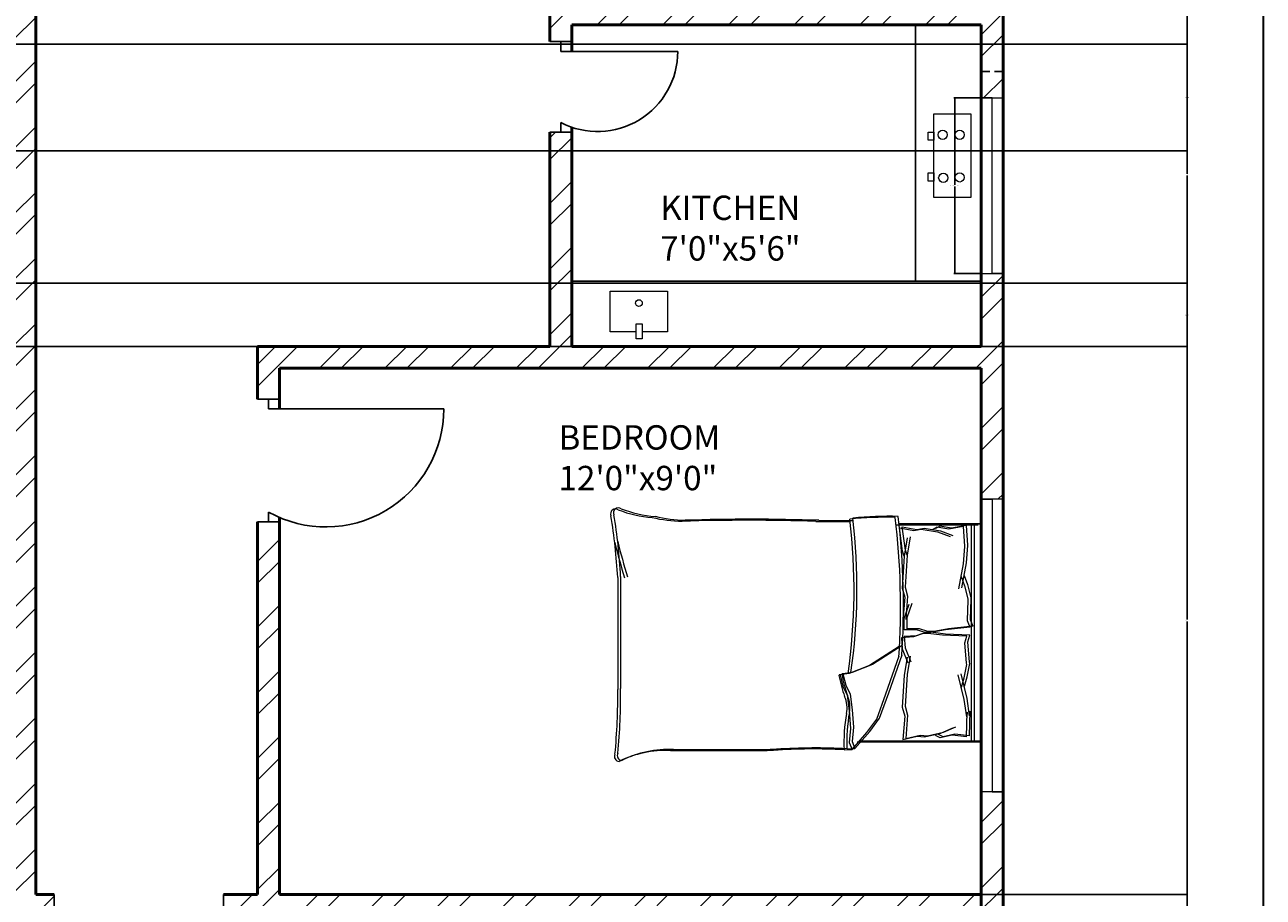
# Model space of a CAD drawing. Units: inches. Extents: x 2129 to 2642, y 1542 to 2414.
# Tile 4 of 9: x 2388 to 2642, y 1828 to 2007. Entities that reach past the tile are written whole.
import ezdxf

# ---------------------------------------------------------------- set-up
doc = ezdxf.new("R2010")
doc.units = ezdxf.units.IN
for name, color, linetype, lineweight in [('A-ANNO-DIMS', 2, 'Continuous', 18), ('A-ANNO-TTLB', 7, 'Continuous', 35), ('A-AREA-IDEN', 7, 'Continuous', 18), ('A-DOOR', 3, 'Continuous', 25), ('A-EQPM', 8, 'Continuous', 18), ('A-FLOR-CASE', 8, 'Continuous', 25), ('A-FLOR-FIXT', 9, 'Continuous', 18), ('A-FURN', 8, 'Continuous', 18), ('A-GLAZ', 4, 'Continuous', 18), ('A-WALL', 7, 'Continuous', 50), ('A-WALL-PATT', 252, 'Continuous', 13)]:
    doc.layers.add(name, color=color, linetype=linetype, lineweight=lineweight)
doc.styles.get("Standard").update_dxf_attribs({"font": 'arial.ttf'})
doc.dimstyles.get("Standard").update_dxf_attribs({"dimtxt": 0.18, "dimasz": 0.18, "dimexe": 0.18, "dimexo": 0.0625, "dimgap": 0.09, "dimtad": 0, "dimtih": 1, "dimtoh": 1, "dimdec": 4, "dimzin": 0, "dimdsep": 46, "dimtxsty": 'Standard', "dimcen": 0.09, "dimadec": 0, "dimazin": 0, "dimtfac": 1, "dimtdec": 4, "dimtofl": 0, "dimtmove": 0, "dimatfit": 3, "dimfxl": 1, "dimtolj": 1, "dimtzin": 0, "dimarcsym": 0})

# ---------------------------------------------------------------- blocks, each defined once
blk = doc.blocks.new('BED-DOUBLE')
for p, q in [((3.24, 59.14), (3.24, 76.05)), ((3.24, 74.61), (47.87, 74.61)), ((3.25, 59.14), (3.25, 76.05)), ((3.25, 74.61), (47.87, 74.61)), ((48.08, 76.05), (3.46, 76.05)), ((3.46, 58.54), (3.46, 75.45)), ((3.46, 58.54), (3.46, 75.45)), ((3.46, 74.02), (48.08, 74.02)), ((3.46, 74.02), (48.08, 74.02)), ((15.76, 73.22), (18.46, 73.9)), ((15.76, 73.22), (18.46, 73.9)), ((18.46, 73.9), (18.76, 73.9)), ((18.46, 73.9), (18.76, 73.9)), ((18.76, 73.9), (22.91, 73.76)), ((18.76, 73.9), (22.91, 73.76)), ((22.91, 73.76), (24.26, 74.3)), ((22.91, 73.76), (24.26, 74.3)), ((23.12, 73.16), (24.47, 73.7)), ((23.12, 73.16), (24.47, 73.7)), ((24.26, 74.3), (24.8, 69.31)), ((24.26, 74.3), (24.8, 69.31)), ((24.47, 73.7), (25.01, 68.71)), ((24.47, 73.7), (25.01, 68.71)), ((26.12, 73.72), (25.9, 68.7)), ((26.12, 73.72), (25.9, 68.7)), ((27.5, 73.27), (26.12, 73.72)), ((27.5, 73.27), (26.12, 73.72)), ((46.79, 73.66), (41.75, 73.75)), ((41.75, 73.75), (42.68, 73.67)), ((46.79, 73.66), (41.75, 73.75)), ((41.75, 73.75), (42.68, 73.67)), ((47.87, 76.05), (47.87, 51.2)), ((47.87, 76.05), (47.87, 51.2)), ((48.08, 76.05), (48.08, 75.45)), ((48.08, 75.45), (48.08, 50.6)), ((48.08, 75.45), (48.08, 50.6)), ((3.64, 72.93), (7.64, 73.24)), ((3.64, 72.93), (7.64, 73.24)), ((3.64, 72.95), (4.18, 69.98)), ((3.64, 72.95), (4.18, 69.98)), ((3.85, 72.33), (7.85, 72.64)), ((3.85, 72.33), (7.85, 72.64)), ((3.85, 72.35), (4.39, 69.38)), ((3.85, 72.35), (4.39, 69.38)), ((7.64, 73.24), (7.74, 73.22)), ((7.64, 73.24), (7.74, 73.22)), ((7.74, 73.22), (11.31, 72.95)), ((7.74, 73.22), (11.31, 72.95)), ((7.85, 72.64), (7.95, 72.62)), ((7.85, 72.64), (7.95, 72.62)), ((7.95, 72.62), (11.52, 72.35)), ((7.95, 72.62), (11.52, 72.35)), ((11.31, 72.95), (16.44, 72.01)), ((11.31, 72.95), (16.44, 72.01)), ((11.52, 72.35), (16.65, 71.41)), ((11.52, 72.35), (16.65, 71.41)), ((13.87, 72.55), (15.76, 73.22)), ((13.87, 72.55), (15.76, 73.22)), ((14.08, 71.95), (15.97, 72.62)), ((14.08, 71.95), (15.97, 72.62)), ((15.97, 72.62), (18.67, 73.3)), ((15.97, 72.62), (18.67, 73.3)), ((18.67, 73.3), (18.97, 73.3)), ((18.67, 73.3), (18.97, 73.3)), ((18.97, 73.3), (23.12, 73.16)), ((18.97, 73.3), (23.12, 73.16)), ((26.34, 73.12), (26.11, 68.1)), ((26.34, 73.12), (26.11, 68.1)), ((27.72, 72.67), (26.34, 73.12)), ((27.72, 72.67), (26.34, 73.12)), ((31.64, 73.66), (27.5, 73.27)), ((31.64, 73.66), (27.5, 73.27)), ((31.85, 73.06), (27.72, 72.67)), ((31.85, 73.06), (27.72, 72.67)), ((31.94, 73.68), (31.64, 73.66)), ((31.94, 73.68), (31.64, 73.66)), ((32.15, 73.08), (31.85, 73.06)), ((32.15, 73.08), (31.85, 73.06)), ((34.68, 73.17), (31.94, 73.68)), ((34.67, 73.17), (31.94, 73.68)), ((34.89, 72.58), (32.15, 73.08)), ((34.89, 72.58), (32.15, 73.08)), ((39.14, 73.18), (34.08, 71.92)), ((39.14, 73.18), (34.08, 71.92)), ((39.35, 72.58), (34.29, 71.32)), ((39.35, 72.58), (34.29, 71.32)), ((36.6, 72.62), (34.67, 73.17)), ((36.6, 72.62), (34.68, 73.17)), ((36.82, 72.02), (34.89, 72.58)), ((36.82, 72.02), (34.89, 72.58)), ((42.68, 73.67), (39.14, 73.18)), ((42.68, 73.67), (39.14, 73.18)), ((42.9, 73.08), (39.35, 72.58)), ((42.9, 73.08), (39.35, 72.58)), ((47.01, 73.06), (41.96, 73.15)), ((41.96, 73.15), (42.9, 73.08)), ((47.01, 73.06), (41.96, 73.15)), ((41.96, 73.15), (42.9, 73.08)), ((46.79, 73.66), (46.44, 70.66)), ((46.79, 73.66), (46.44, 70.66)), ((47.01, 73.06), (46.65, 70.06)), ((47.01, 73.06), (46.65, 70.06)), ((4.18, 69.98), (3.77, 67.55)), ((4.18, 69.98), (3.77, 67.55)), ((4.39, 69.38), (3.98, 66.95)), ((4.39, 69.38), (3.99, 66.95)), ((4.72, 67.69), (5.66, 70.25)), ((4.72, 67.69), (5.66, 70.25)), ((4.93, 67.09), (5.87, 69.65)), ((4.93, 67.09), (5.87, 69.65)), ((24.8, 69.31), (25.34, 66.34)), ((24.8, 69.31), (25.34, 66.34)), ((25.01, 68.71), (25.55, 65.74)), ((25.01, 68.71), (25.55, 65.74)), ((25.9, 68.7), (25.54, 65.7)), ((25.9, 68.7), (25.54, 65.7)), ((46.04, 68.34), (44.94, 70.84)), ((46.04, 68.34), (44.94, 70.84)), ((46.26, 67.74), (45.15, 70.24)), ((46.26, 67.74), (45.15, 70.24)), ((46.44, 70.66), (46.99, 68.26)), ((46.44, 70.66), (46.99, 68.26)), ((46.65, 70.06), (47.21, 67.66)), ((46.65, 70.06), (47.21, 67.66)), ((3.77, 67.55), (4.31, 66.61)), ((3.77, 67.55), (4.31, 66.61)), ((3.98, 66.95), (4.52, 66.01)), ((3.99, 66.95), (4.53, 66.01)), ((4.18, 64.31), (4.72, 67.69)), ((4.18, 64.31), (4.72, 67.69)), ((4.39, 63.71), (4.93, 67.09)), ((4.39, 63.71), (4.93, 67.09)), ((25.34, 66.34), (25.34, 65.12)), ((25.34, 66.34), (25.34, 65.12)), ((26.11, 68.1), (25.76, 65.11)), ((26.11, 68.1), (25.76, 65.11)), ((46.79, 65), (46.04, 68.34)), ((46.79, 65), (46.04, 68.34)), ((47.01, 64.41), (46.26, 67.74)), ((47.01, 64.41), (46.26, 67.74)), ((46.99, 68.26), (46.51, 67.28)), ((46.99, 68.26), (46.51, 67.28)), ((47.21, 67.66), (46.73, 66.69)), ((47.21, 67.66), (46.73, 66.69)), ((4.45, 62.82), (4.18, 64.31)), ((4.45, 62.82), (4.18, 64.31)), ((4.66, 62.23), (4.39, 63.71)), ((4.66, 62.23), (4.39, 63.71)), ((25.34, 65.12), (24.8, 63.36)), ((25.34, 65.12), (24.8, 63.36)), ((25.55, 64.52), (25.01, 62.77)), ((25.55, 64.52), (25.01, 62.77)), ((25.54, 65.7), (25.62, 64.49)), ((25.54, 65.7), (25.62, 64.49)), ((25.55, 65.74), (25.55, 64.52)), ((25.55, 65.74), (25.55, 64.52)), ((25.62, 64.49), (26.27, 62.77)), ((25.62, 64.49), (26.27, 62.77)), ((25.76, 65.11), (25.83, 63.89)), ((25.76, 65.11), (25.83, 63.89)), ((25.83, 63.89), (26.48, 62.18)), ((25.83, 63.89), (26.48, 62.18)), ((46.62, 63.5), (46.79, 65)), ((46.62, 63.5), (46.79, 65)), ((46.83, 62.91), (47.01, 64.41)), ((46.83, 62.91), (47.01, 64.41)), ((3.91, 59.85), (4.45, 62.82)), ((3.91, 59.85), (4.45, 62.82)), ((4.12, 59.26), (4.66, 62.23)), ((4.12, 59.26), (4.66, 62.23)), ((5.96, 61.45), (9.72, 60.83)), ((5.96, 61.45), (9.72, 60.83)), ((22.51, 60.86), (19.57, 61.88)), ((22.51, 60.86), (19.57, 61.88)), ((22.72, 60.26), (19.78, 61.28)), ((22.72, 60.26), (19.78, 61.28)), ((24.8, 63.36), (24.8, 60.86)), ((24.8, 63.36), (24.8, 60.86)), ((25.01, 62.77), (25.01, 60.26)), ((25.01, 62.77), (25.01, 60.26)), ((26.27, 62.77), (26.42, 60.27)), ((26.27, 62.77), (26.42, 60.27)), ((26.48, 62.18), (26.64, 59.68)), ((26.48, 62.18), (26.64, 59.68)), ((28.71, 60.42), (31.58, 61.62)), ((28.71, 60.42), (31.58, 61.62)), ((28.93, 59.82), (31.79, 61.02)), ((28.93, 59.82), (31.79, 61.02)), ((30.41, 61.45), (34.17, 60.83)), ((30.41, 61.45), (34.17, 60.83)), ((47.34, 60.57), (46.62, 63.5)), ((47.34, 60.57), (46.62, 63.5)), ((47.55, 59.98), (46.83, 62.91)), ((47.55, 59.98), (46.83, 62.91)), ((8.67, 60.53), (3.91, 59.85)), ((8.67, 60.53), (3.91, 59.85)), ((8.88, 59.93), (4.12, 59.26)), ((8.88, 59.93), (4.12, 59.26)), ((6.17, 60.86), (9.94, 60.23)), ((6.17, 60.86), (9.94, 60.23)), ((9.72, 60.83), (8.67, 60.53)), ((9.72, 60.83), (8.67, 60.53)), ((9.94, 60.23), (8.88, 59.93)), ((9.94, 60.23), (8.88, 59.93)), ((9.72, 60.83), (16.27, 60.43)), ((9.72, 60.83), (16.27, 60.43)), ((9.94, 60.23), (16.48, 59.83)), ((9.94, 60.23), (16.48, 59.83)), ((16.27, 60.43), (18.1, 60.95)), ((16.27, 60.43), (18.1, 60.95)), ((16.48, 59.83), (18.31, 60.35)), ((16.48, 59.83), (18.31, 60.35)), ((18.1, 60.95), (22.89, 60.57)), ((18.1, 60.95), (22.89, 60.57)), ((18.31, 60.35), (23.11, 59.98)), ((18.31, 60.35), (23.1, 59.98)), ((24.8, 60.86), (22.51, 60.86)), ((24.8, 60.86), (22.51, 60.86)), ((25.01, 60.26), (22.72, 60.26)), ((25.01, 60.26), (22.72, 60.26)), ((26.42, 60.27), (28.71, 60.42)), ((26.42, 60.27), (28.71, 60.42)), ((26.64, 59.68), (28.93, 59.82)), ((26.64, 59.68), (28.93, 59.82)), ((28.25, 59.82), (32.17, 53.75)), ((28.25, 59.82), (32.17, 53.75)), ((28.47, 59.22), (32.38, 53.16)), ((28.47, 59.22), (32.38, 53.16)), ((37.95, 57.08), (30.17, 59.82)), ((37.95, 57.08), (30.17, 59.82)), ((38.16, 56.48), (30.38, 59.22)), ((38.16, 56.48), (30.38, 59.22)), ((30.62, 60.86), (34.39, 60.23)), ((30.62, 60.86), (34.38, 60.23)), ((34.17, 60.83), (40.72, 60.43)), ((34.17, 60.83), (40.72, 60.43)), ((34.38, 60.23), (40.93, 59.83)), ((34.39, 60.23), (40.93, 59.83)), ((40.72, 60.43), (42.55, 60.95)), ((40.72, 60.43), (42.55, 60.95)), ((40.93, 59.83), (42.76, 60.35)), ((40.93, 59.83), (42.76, 60.35)), ((42.55, 60.95), (47.34, 60.57)), ((42.55, 60.95), (47.34, 60.57)), ((42.76, 60.35), (47.55, 59.98)), ((42.76, 60.35), (47.55, 59.98)), ((43.16, 55.2), (37.95, 57.08)), ((43.16, 55.2), (37.95, 57.08)), ((43.37, 54.6), (38.16, 56.48)), ((43.37, 54.6), (38.16, 56.48)), ((32.17, 53.75), (33.76, 49.56)), ((32.17, 53.75), (33.76, 49.56)), ((45.91, 53.17), (43.16, 55.2)), ((45.91, 53.17), (43.16, 55.2)), ((46.12, 52.58), (43.37, 54.6)), ((46.12, 52.58), (43.37, 54.6)), ((32.38, 53.16), (33.97, 48.96)), ((32.38, 53.16), (33.97, 48.96)), ((49.37, 50.14), (45.91, 53.17)), ((49.36, 50.14), (45.91, 53.17)), ((49.58, 49.54), (46.12, 52.58)), ((49.58, 49.54), (46.12, 52.58)), ((33.76, 49.56), (34.05, 47.68)), ((33.76, 49.56), (34.05, 47.68)), ((33.97, 48.96), (34.26, 47.09)), ((33.97, 48.96), (34.26, 47.09)), ((36.36, 48.26), (38.24, 49.13)), ((36.36, 48.26), (38.24, 49.13)), ((36.57, 47.66), (38.45, 48.53)), ((36.57, 47.66), (38.45, 48.53)), ((38.24, 49.13), (41.42, 49.56)), ((38.24, 49.13), (41.42, 49.56)), ((38.45, 48.53), (41.64, 48.96)), ((38.45, 48.53), (41.64, 48.96)), ((41.42, 49.56), (45.04, 49.85)), ((41.42, 49.56), (45.04, 49.85)), ((41.64, 48.96), (45.25, 49.25)), ((41.64, 48.96), (45.25, 49.25)), ((45.04, 49.85), (47.93, 49.56)), ((45.04, 49.85), (47.93, 49.56)), ((45.25, 49.25), (48.14, 48.96)), ((45.25, 49.25), (48.14, 48.96)), ((47.93, 49.56), (49.37, 50.14)), ((47.93, 49.56), (49.36, 50.14)), ((48.14, 48.96), (49.58, 49.54)), ((48.14, 48.96), (49.58, 49.54)), ((49.44, 48.51), (49.36, 50.14, 3.61)), ((49.44, 48.51), (49.37, 50.14, 3.61)), ((49.65, 47.91), (49.58, 49.54, 3.61)), ((49.65, 47.91), (49.58, 49.54, 3.61)), ((34.05, 47.68), (36.36, 48.26)), ((34.05, 47.68), (36.36, 48.26)), ((34.26, 47.09), (36.57, 47.66)), ((34.26, 47.09), (36.57, 47.66)), ((14.07, 2.05), (37.05, 2.05)), ((14.07, 2.05), (37.05, 2.05)), ((14.28, 1.46), (37.26, 1.46)), ((14.28, 1.46), (37.26, 1.46))]:
    blk.add_line(p, q)
for centre, radius, start, end in [((79.52, 57.28), 77.79, 178.7218, 185.604), ((79.52, 57.28), 77.79, 178.7218, 185.604), ((19.94, -93.94), 154.04, 86.0865, 96.7821), ((19.94, -93.94), 154.04, 86.0865, 96.7821), ((20.16, -94.54), 154.04, 86.0865, 96.7821), ((20.16, -94.54), 154.04, 86.0865, 96.7821), ((79.73, 56.69), 77.79, 178.7218, 185.604), ((79.73, 56.69), 77.79, 178.7218, 185.604), ((16.58, -69.91), 120.47, 81.7845, 96.9006), ((16.58, -69.91), 120.47, 81.7845, 96.9006), ((16.79, -70.51), 120.47, 81.7845, 96.9006), ((16.79, -70.51), 120.47, 81.7845, 96.9006), ((-156.22, 46.94), 158.84, 358.4762, 1.0082), ((-156.22, 46.94), 158.84, 358.4762, 1.0082), ((-156.01, 46.34), 158.84, 358.4762, 1.0082), ((-156.01, 46.34), 158.84, 358.4762, 1.0082), ((29.09, 74.66), 27.69, 280.6617, 289.8806), ((29.09, 74.66), 27.69, 280.6617, 289.8806), ((40.85, 43.3), 5.81, 78.6608, 113.7384), ((40.85, 43.3), 5.81, 78.6608, 113.7384), ((41.06, 42.71), 5.81, 78.6608, 113.7384), ((41.06, 42.71), 5.81, 78.6608, 113.7384), ((47.93, 82.26), 33.79, 259.8763, 272.5657), ((47.93, 82.26), 33.79, 259.8763, 272.5657), ((48.14, 81.67), 33.79, 259.8763, 272.5657), ((48.14, 81.67), 33.79, 259.8763, 272.5657), ((170.19, 42.14), 120.92, 176.9791, 183.8365), ((170.19, 42.14), 120.92, 176.9791, 183.8365), ((34.21, 47.62), 0.172, 160.2464, 271.1377), ((34.21, 47.62), 0.172, 160.2464, 271.1377), ((34.42, 47.03), 0.172, 160.2464, 271.1377), ((34.42, 47.03), 0.172, 160.2464, 271.1377), ((29.3, 74.07), 27.69, 280.6617, 289.8806), ((29.3, 74.07), 27.69, 280.6617, 289.8806), ((170.4, 41.54), 120.92, 176.9791, 183.8365), ((170.4, 41.54), 120.92, 176.9791, 183.8365), ((452.7, 28.79), 450.36, 178.2277, 181.7185), ((452.7, 28.79), 450.36, 178.2277, 181.7185), ((452.91, 28.19), 450.36, 178.2277, 181.7185), ((452.91, 28.19), 450.36, 178.2277, 181.7185), ((-4210.02, 12.72), 4259.62, 0.00217, 0.28689), ((-4210.02, 12.72), 4259.62, 0.00217, 0.28689), ((-4209.81, 12.12), 4259.62, 0.00217, 0.28689), ((-4209.81, 12.12), 4259.62, 0.00217, 0.28689), ((-25.12, 15.81), 27.67, 346.0648, 358.9113), ((-25.12, 15.81), 27.67, 346.0648, 358.9113), ((-24.9, 15.21), 27.67, 346.0648, 358.9113), ((-24.9, 15.21), 27.67, 346.0648, 358.9113), ((71.11, 11.93), 21.54, 177.4714, 206.4681), ((71.11, 11.93), 21.54, 177.4714, 206.4681), ((71.33, 11.33), 21.54, 177.4714, 206.4681), ((71.32, 11.33), 21.54, 177.4714, 206.4681), ((-20.22, 10.43), 22, 337.9751, 356.652), ((-20.22, 10.43), 22, 337.9751, 356.652), ((-20.01, 9.83), 22, 337.9751, 356.652), ((-20.01, 9.83), 22, 337.9751, 356.652), ((-16.08, 98.19), 99.41, 283.3832, 287.7053), ((-16.08, 98.19), 99.41, 283.3832, 287.7053), ((-15.87, 97.59), 99.41, 283.3832, 287.7053), ((-15.87, 97.59), 99.41, 283.3832, 287.7053), ((1.02, 1.61), 1.02, 146.1736, 293.4781), ((1.02, 1.61), 1.02, 146.1736, 293.4781), ((1.23, 1.01), 1.02, 146.1736, 293.4781), ((1.23, 1.01), 1.02, 146.1736, 293.4781), ((20.01, -111.48), 113.69, 92.9958, 99.4091), ((20.01, -111.48), 113.69, 92.9958, 99.4091), ((20.22, -112.08), 113.69, 92.9958, 99.4091), ((20.22, -112.08), 113.69, 92.9958, 99.4091), ((38.43, -122.17), 124.23, 84.4998, 90.6351), ((38.43, -122.17), 124.23, 84.4998, 90.6351), ((38.64, -122.76), 124.23, 84.4998, 90.6351), ((38.64, -122.76), 124.23, 84.4998, 90.6351), ((50.81, 2.4), 1.03, 242.6588, 356.02), ((50.81, 2.4), 1.03, 242.6588, 356.02), ((51.02, 1.81), 1.03, 242.6588, 356.02), ((51.02, 1.81), 1.03, 242.6588, 356.02)]:
    blk.add_arc(centre, radius, start, end)
blk = doc.blocks.new('COOKTOP-4-BURNER')
for points in [[(0, 17.17), (7.64, 17.17), (7.64, 0), (0, 0)], [(7.64, 13.8), (8.8, 13.8), (8.8, 12.1), (7.64, 12.1)], [(7.64, 5.39), (8.8, 5.39), (8.8, 3.7), (7.64, 3.7)]]:
    blk.add_lwpolyline(points, close=True)
for centre in [(2.31, 13.01), (5.67, 13.11), (2.31, 4.27), (5.8, 4.27)]:
    blk.add_circle(centre, 0.951)
blk = doc.blocks.new('SINK-KITCHEN')
blk.add_lwpolyline([(5.28, 1.49), (0, 1.49), (0, 9.84), (11.71, 9.84), (11.71, 1.49), (6.54, 1.49)])
blk.add_lwpolyline([(5.28, 3.09), (6.54, 3.09), (6.54, 0), (5.28, 0)], close=True)
blk.add_circle((5.88, 7.38), 0.679)
blk = doc.blocks.new('WIN-60-A')
for p, q in [((0, 4.5), (0, 0)), ((60, 2.25), (60, 4.5)), ((60, 4.5), (60, 0)), ((0, 0), (0, 2.25)), ((0, 2.25), (60, 2.25))]:
    blk.add_line(p, q)
blk = doc.blocks.new('WIN-36')
for p, q in [((4.5, 36), (0, 36)), ((0, 36), (2.25, 36)), ((2.25, 36), (2.25, 0)), ((4.5, 0), (0, 0)), ((2.25, 0), (4.5, 0))]:
    blk.add_line(p, q)
blk = doc.blocks.new('*D18')
at = {"layer": 'A-ANNO-DIMS', "color": 0, "lineweight": -2, "transparency": 16777216}
for p, q in [((2584.34, 1992.2), (2578.82, 1992.2)), ((2579, 1992.02), (2579, 1974.38)), ((2579, 1956.38), (2579, 1974.02)), ((2584.34, 1956.2), (2578.82, 1956.2))]:
    blk.add_line(p, q, dxfattribs=at)
at = {"layer": 'A-ANNO-DIMS', "color": 0, "transparency": 16777216}
for points in [[(2578.97, 1992.02), (2579.03, 1992.02), (2579, 1992.2)], [(2578.97, 1956.38), (2579.03, 1956.38), (2579, 1956.2)]]:
    blk.add_solid(points, dxfattribs=at)
at = {"layer": 'Defpoints', "color": 0, "transparency": 16777216}
for p in [(2584.4, 1992.2), (2579, 1956.2), (2584.4, 1956.2)]:
    blk.add_point(p, dxfattribs=at)
at = {"layer": 'A-ANNO-DIMS', "color": 0, "transparency": 16777216, "insert": (2579, 1974.2), "char_height": 0.18, "attachment_point": 5}
blk.add_mtext('\\A1;WINDOW 36 TYP.', dxfattribs=at)
blk = doc.blocks.new('*D19')
at = {"layer": 'A-ANNO-DIMS', "color": 0, "lineweight": -2, "transparency": 16777216}
for p, q in [((2584.4, 1992.26), (2584.4, 1997.78)), ((2584.58, 1997.6), (2586.2, 1997.6)), ((2588.72, 1997.6), (2587.11, 1997.6)), ((2588.9, 1992.26), (2588.9, 1997.78))]:
    blk.add_line(p, q, dxfattribs=at)
at = {"layer": 'A-ANNO-DIMS', "color": 0, "transparency": 16777216}
for points in [[(2584.58, 1997.63), (2584.58, 1997.57), (2584.4, 1997.6)], [(2588.72, 1997.63), (2588.72, 1997.57), (2588.9, 1997.6)]]:
    blk.add_solid(points, dxfattribs=at)
at = {"layer": 'Defpoints', "color": 0, "transparency": 16777216}
for p in [(2584.4, 1997.6), (2584.4, 1992.2), (2588.9, 1992.2)]:
    blk.add_point(p, dxfattribs=at)
at = {"layer": 'A-ANNO-DIMS', "color": 0, "transparency": 16777216, "insert": (2586.65, 1997.6), "char_height": 0.18, "attachment_point": 5}
blk.add_mtext('\\A1;5 TYP.', dxfattribs=at)
blk = doc.blocks.new('*D40')
at = {"layer": 'A-ANNO-DIMS', "color": 0, "lineweight": -2, "transparency": 16777216}
for p, q in [((2584.47, 1828.72), (2626.83, 1828.72)), ((2626.65, 1828.54), (2626.65, 1764.4)), ((2626.65, 1699.9), (2626.65, 1764.04)), ((2588.97, 1699.72), (2626.83, 1699.72))]:
    blk.add_line(p, q, dxfattribs=at)
at = {"layer": 'A-ANNO-DIMS', "color": 0, "transparency": 16777216}
for points in [[(2626.62, 1828.54), (2626.68, 1828.54), (2626.65, 1828.72)], [(2626.62, 1699.9), (2626.68, 1699.9), (2626.65, 1699.72)]]:
    blk.add_solid(points, dxfattribs=at)
at = {"layer": 'Defpoints', "color": 0, "transparency": 16777216}
for p in [(2584.4, 1828.72), (2626.65, 1828.72), (2588.9, 1699.72)]:
    blk.add_point(p, dxfattribs=at)
at = {"layer": 'A-ANNO-DIMS', "color": 0, "transparency": 16777216, "insert": (2626.65, 1764.22), "char_height": 0.18, "attachment_point": 5}
blk.add_mtext('\\A1;129', dxfattribs=at)
blk = doc.blocks.new('*D41')
at = {"layer": 'A-ANNO-DIMS', "color": 0, "lineweight": -2, "transparency": 16777216}
for p, q in [((2584.47, 1941.22), (2626.83, 1941.22)), ((2626.65, 1941.04), (2626.65, 1885.15)), ((2626.65, 1828.9), (2626.65, 1884.79)), ((2584.47, 1828.72), (2626.83, 1828.72))]:
    blk.add_line(p, q, dxfattribs=at)
at = {"layer": 'A-ANNO-DIMS', "color": 0, "transparency": 16777216}
for points in [[(2626.62, 1941.04), (2626.68, 1941.04), (2626.65, 1941.22)], [(2626.62, 1828.9), (2626.68, 1828.9), (2626.65, 1828.72)]]:
    blk.add_solid(points, dxfattribs=at)
at = {"layer": 'Defpoints', "color": 0, "transparency": 16777216}
for p in [(2584.4, 1941.22), (2626.65, 1941.22), (2584.4, 1828.72)]:
    blk.add_point(p, dxfattribs=at)
at = {"layer": 'A-ANNO-DIMS', "color": 0, "transparency": 16777216, "insert": (2626.65, 1884.97), "char_height": 0.18, "attachment_point": 5}
blk.add_mtext('\\A1;112.5', dxfattribs=at)
blk = doc.blocks.new('*D42')
at = {"layer": 'A-ANNO-DIMS', "color": 0, "lineweight": -2, "transparency": 16777216}
for p, q in [((2584.47, 2011.72), (2626.83, 2011.72)), ((2626.65, 2011.54), (2626.65, 1976.65)), ((2626.65, 1941.4), (2626.65, 1976.29)), ((2584.47, 1941.22), (2626.83, 1941.22))]:
    blk.add_line(p, q, dxfattribs=at)
at = {"layer": 'A-ANNO-DIMS', "color": 0, "transparency": 16777216}
for points in [[(2626.62, 2011.54), (2626.68, 2011.54), (2626.65, 2011.72)], [(2626.62, 1941.4), (2626.68, 1941.4), (2626.65, 1941.22)]]:
    blk.add_solid(points, dxfattribs=at)
at = {"layer": 'Defpoints', "color": 0, "transparency": 16777216}
for p in [(2584.4, 2011.72), (2626.65, 2011.72), (2584.4, 1941.22)]:
    blk.add_point(p, dxfattribs=at)
at = {"layer": 'A-ANNO-DIMS', "color": 0, "transparency": 16777216, "insert": (2626.65, 1976.47), "char_height": 0.18, "attachment_point": 5}
blk.add_mtext('\\A1;70.5', dxfattribs=at)
blk = doc.blocks.new('*D47')
at = {"layer": 'A-ANNO-DIMS', "color": 0, "lineweight": -2, "transparency": 16777216}
for p, q in [((2279.97, 2003.23), (2626.83, 2003.23)), ((2626.65, 2003.05), (2626.65, 1992.47)), ((2626.65, 1981.52), (2626.65, 1992.1)), ((2279.97, 1981.34), (2626.83, 1981.34))]:
    blk.add_line(p, q, dxfattribs=at)
at = {"layer": 'A-ANNO-DIMS', "color": 0, "transparency": 16777216}
for points in [[(2626.62, 2003.05), (2626.68, 2003.05), (2626.65, 2003.23)], [(2626.62, 1981.52), (2626.68, 1981.52), (2626.65, 1981.34)]]:
    blk.add_solid(points, dxfattribs=at)
at = {"layer": 'Defpoints', "color": 0, "transparency": 16777216}
for p in [(2279.9, 2003.23), (2626.65, 2003.23), (2279.9, 1981.34)]:
    blk.add_point(p, dxfattribs=at)
at = {"layer": 'A-ANNO-DIMS', "color": 0, "transparency": 16777216, "insert": (2626.65, 1992.29), "char_height": 0.18, "attachment_point": 5}
blk.add_mtext('\\A1;21.886', dxfattribs=at)
blk = doc.blocks.new('*D49')
at = {"layer": 'A-ANNO-DIMS', "color": 0, "lineweight": -2, "transparency": 16777216}
for p, q in [((2275.47, 1954.17), (2626.83, 1954.17)), ((2626.65, 1953.99), (2626.65, 1947.88)), ((2626.65, 1941.4), (2626.65, 1947.52)), ((2275.47, 1941.22), (2626.83, 1941.22))]:
    blk.add_line(p, q, dxfattribs=at)
at = {"layer": 'A-ANNO-DIMS', "color": 0, "transparency": 16777216}
for points in [[(2626.62, 1953.99), (2626.68, 1953.99), (2626.65, 1954.17)], [(2626.62, 1941.4), (2626.68, 1941.4), (2626.65, 1941.22)]]:
    blk.add_solid(points, dxfattribs=at)
at = {"layer": 'Defpoints', "color": 0, "transparency": 16777216}
for p in [(2275.4, 1954.17), (2626.65, 1954.17), (2275.4, 1941.22)]:
    blk.add_point(p, dxfattribs=at)
at = {"layer": 'A-ANNO-DIMS', "color": 0, "transparency": 16777216, "insert": (2626.65, 1947.7), "char_height": 0.18, "attachment_point": 5}
blk.add_mtext('\\A1;12.953', dxfattribs=at)

msp = doc.modelspace()

# ---------------------------------------------------------------- hatches: boundary and pattern name
at = {"layer": 'A-WALL-PATT'}
h = msp.add_hatch(dxfattribs=at)
h.set_pattern_fill('ANSI32', color=256)
h.paths.add_polyline_path([(2306.2606, 2305.9717), (2306.2606, 2308.2217), (2276.3515, 2308.2217), (2276.3515, 2303.7217), (2306.2606, 2303.7217)])
h.paths.add_polyline_path([(2216.3515, 2305.9717), (2216.3515, 2308.2217), (2186.9043, 2308.2217), (2186.9043, 2278.1696), (2191.4043, 2278.1696), (2191.4043, 2303.7217), (2216.3515, 2303.7217)])
h.paths.add_polyline_path([(2339.9043, 2335.7217), (2362.1938, 2335.7217), (2362.1938, 2340.2217), (2335.4043, 2340.2217), (2335.4043, 2308.2217), (2329.3487, 2308.2217), (2329.3487, 2305.9717), (2329.3487, 2303.7217), (2335.4043, 2303.7217), (2335.4043, 2186.7217), (2329.4345, 2186.7217), (2329.4345, 2182.2217), (2335.4043, 2182.2217), (2335.4043, 2174.7178), (2339.9043, 2174.7178), (2339.9043, 2182.2217), (2339.9043, 2303.7217)])
h.paths.add_polyline_path([(2440.4043, 2340.2217), (2411.654, 2340.2217), (2411.654, 2335.7217), (2435.9043, 2335.7217), (2435.9043, 2303.7217), (2435.9043, 2182.2217), (2435.9043, 2174.1935), (2438.1543, 2174.1935), (2440.4043, 2174.1935), (2440.4043, 2182.2217), (2444.653, 2182.2217), (2444.653, 2184.4717), (2444.653, 2186.7217), (2440.4043, 2186.7217), (2440.4043, 2303.7217), (2445.8547, 2303.7217), (2445.8547, 2308.2217), (2440.4043, 2308.2217)])
h.paths.add_polyline_path([(2498.2381, 2308.2217), (2470.3901, 2308.2217), (2470.3901, 2303.7217), (2498.2381, 2303.7217), (2498.2381, 2305.9717)])
h.paths.add_polyline_path([(2588.9043, 2308.2217), (2586.9043, 2308.2217), (2558.2381, 2308.2217), (2558.2381, 2303.7217), (2584.4043, 2303.7217), (2584.4043, 2279.1087), (2588.9043, 2279.1087)])
h.paths.add_polyline_path([(2588.9043, 2219.1087), (2584.4043, 2219.1087), (2584.4043, 2186.7217), (2478.0667, 2186.7217), (2478.0667, 2182.2217), (2584.4043, 2182.2217), (2584.4043, 2157.7883), (2588.9043, 2157.7883)])
h.paths.add_polyline_path([(2588.9043, 2097.7883), (2584.6063, 2097.7883), (2584.6063, 2075.5462, -0.09241561), (2584.4043, 2074.4627), (2584.4043, 2064.2217), (2495.9043, 2064.2217), (2495.9043, 2040.4611), (2500.4043, 2040.4611), (2500.4043, 2059.7217), (2584.4043, 2059.7217), (2584.4043, 2052.2164), (2588.9043, 2052.2164)])
h.paths.add_polyline_path([(2588.9043, 2028.2164), (2584.4043, 2028.2164), (2584.4043, 2011.7217), (2500.4043, 2011.7217), (2500.4043, 2015.243), (2498.1543, 2015.243), (2495.9043, 2015.243), (2495.9043, 2007.2217), (2495.9043, 2003.7597), (2500.4043, 2003.7597), (2500.4043, 2007.2217), (2584.4043, 2007.2217), (2584.4043, 1992.1997), (2588.9043, 1992.1997)])
h.paths.add_polyline_path([(2588.9043, 1956.1997), (2584.4043, 1956.1997), (2584.4043, 1941.2217), (2500.4043, 1941.2217), (2500.4043, 1985.1493), (2498.1543, 1985.1493), (2495.9043, 1985.1493), (2495.9043, 1941.2217), (2435.9043, 1941.2217), (2435.9043, 1930.3963), (2440.4043, 1930.3963), (2440.4043, 1936.7217), (2584.4043, 1936.7217), (2584.4043, 1909.8406), (2588.9043, 1909.8406)])
h.paths.add_polyline_path([(2588.9043, 1849.8406), (2584.4043, 1849.8406), (2584.4043, 1801.3526), (2588.9043, 1801.3526)])
h.paths.add_polyline_path([(2584.4043, 1828.7217), (2495.9043, 1828.7217), (2440.4043, 1828.7217), (2440.4043, 1905.2159), (2438.1543, 1905.2159), (2435.9043, 1905.2159), (2435.9043, 1828.7217), (2428.9101, 1828.7217), (2428.9101, 1824.2217), (2584.4043, 1824.2217)])
h.paths.add_polyline_path([(2588.9043, 1741.3526), (2584.4043, 1741.3526), (2584.4043, 1704.2217), (2468.3173, 1704.2217), (2468.3173, 1701.9717), (2468.3173, 1699.7217), (2588.9043, 1699.7217)])
h.paths.add_polyline_path([(2442.4043, 1761.7217), (2435.0216, 1761.7217), (2435.0216, 1757.2217), (2437.9043, 1757.2217), (2437.9043, 1665.7217), (2442.4043, 1665.7217), (2442.4043, 1667.7217), (2442.4043, 1699.7217), (2446.6907, 1699.7217), (2446.6907, 1701.9717), (2446.6907, 1704.2217), (2442.4043, 1704.2217)])
h.paths.add_polyline_path([(2390.4043, 1757.2217), (2410.8996, 1757.2217), (2410.8996, 1761.7217), (2360.1741, 1761.7217), (2360.1741, 1759.4717), (2360.1741, 1757.2217), (2385.9043, 1757.2217), (2385.9043, 1674.8326), (2390.4043, 1674.8326)])
h.paths.add_polyline_path([(2337.9043, 1757.2217), (2340.3592, 1757.2217), (2340.3592, 1759.4717), (2340.3592, 1761.7217), (2333.4043, 1761.7217), (2333.4043, 1704.2217), (2327.381, 1704.2217), (2327.381, 1701.9717), (2327.381, 1699.7217), (2333.4043, 1699.7217), (2333.4043, 1665.7217), (2337.9043, 1665.7217)])
h.paths.add_polyline_path([(2191.4043, 1743.4804), (2186.9043, 1743.4804), (2186.9043, 1699.7217), (2188.9043, 1699.7217), (2191.4043, 1699.7217), (2306.5617, 1699.7217), (2306.5617, 1704.2217), (2191.4043, 1704.2217)])
h.paths.add_polyline_path([(2191.4043, 1859.8992), (2186.9043, 1859.8992), (2186.9043, 1803.4804), (2189.1543, 1803.4804), (2191.4043, 1803.4804)])
h.paths.add_polyline_path([(2352.5445, 1828.7217), (2191.4043, 1828.7217), (2191.4043, 1824.2217), (2333.4043, 1824.2217), (2352.5445, 1824.2217), (2352.5445, 1826.4717)])
h.paths.add_polyline_path([(2390.4043, 2085.328), (2385.9043, 2085.328), (2385.9043, 1828.7217), (2381.9668, 1828.7217), (2381.9668, 1826.4717), (2381.9668, 1824.2217), (2385.9043, 1824.2217), (2385.9043, 1761.7217), (2390.4043, 1761.7217), (2390.4043, 1824.2217), (2394.1868, 1824.2217), (2394.1868, 1827.6339), (2394.1868, 1828.7217), (2390.4043, 1828.7217)])
h.paths.add_polyline_path([(2339.9043, 1941.2217), (2335.4043, 1941.2217), (2279.9043, 1941.2217), (2279.9043, 1981.3432), (2277.6543, 1981.3432), (2275.4043, 1981.3432), (2275.4043, 1941.2217), (2191.4043, 1941.2217), (2191.4043, 1958.1079), (2186.9043, 1958.1079), (2186.9043, 1919.8992), (2189.1543, 1919.8992), (2191.4043, 1919.8992), (2191.4043, 1936.7217), (2279.9043, 1936.7217), (2335.4043, 1936.7217), (2335.4043, 1931.1382), (2339.9043, 1931.1382)])
h.paths.add_polyline_path([(2339.9043, 1902.7544), (2337.6543, 1902.7544), (2335.4043, 1902.7544), (2335.4043, 1828.7217), (2339.9043, 1828.7217)])
h.paths.add_polyline_path([(2279.9043, 2015.263), (2277.6543, 2015.263), (2275.4043, 2015.263), (2275.4043, 2011.7217), (2191.4043, 2011.7217), (2191.4043, 2026.6781), (2186.9043, 2026.6781), (2186.9043, 1994.1079), (2189.1543, 1994.1079), (2191.4043, 1994.1079), (2191.4043, 2007.2217), (2275.4043, 2007.2217), (2275.4043, 2003.2288), (2279.9043, 2003.2288), (2279.9043, 2007.2217)])
h.paths.add_polyline_path([(2296.0216, 2186.7217), (2191.4043, 2186.7217), (2191.4043, 2218.1696), (2186.9043, 2218.1696), (2186.9043, 2158.4509), (2191.4043, 2158.4509), (2191.4043, 2182.2217), (2296.0216, 2182.2217), (2296.0216, 2184.4717)])
h.paths.add_polyline_path([(2191.4043, 2098.4509), (2189.1543, 2098.4509), (2186.9043, 2098.4509), (2186.9043, 2050.6781), (2189.0487, 2050.6781), (2191.4043, 2050.6781), (2191.4043, 2059.7217), (2275.4043, 2059.7217), (2275.4043, 2038.4133), (2279.9043, 2038.4133), (2279.9043, 2064.2217), (2191.4043, 2064.2217)])
h.paths.add_polyline_path([(2268.3923, 1605.9386), (2516.3159, 1605.9386), (2516.3159, 1643.0314), (2268.3923, 1643.0314)], flags=9)
h.paths.add_polyline_path([(2399.6079, 1710.4489), (2428.8405, 1710.4489), (2428.8405, 1729.1062), (2399.6079, 1729.1062)], flags=9)
h.paths.add_polyline_path([(2342.1483, 1708.9956), (2371.3809, 1708.9956), (2371.3809, 1727.653), (2342.1483, 1727.653)], flags=9)
h.paths.add_polyline_path([(2200.7404, 1677.2519), (2282.3059, 1677.2519), (2282.3059, 1687.5555), (2200.7404, 1687.5555)], flags=9)
h.paths.add_polyline_path([(2209.8153, 1704.7448), (2250.627, 1704.7448), (2250.627, 1723.4021), (2209.8153, 1723.4021)], flags=25)
h.paths.add_polyline_path([(2213.9996, 1911.284), (2252.84, 1911.284), (2252.84, 1929.9413), (2213.9996, 1929.9413)], flags=9)
h.paths.add_polyline_path([(2210.8865, 1962.0987), (2244.0447, 1962.0987), (2244.0447, 1980.7561), (2210.8865, 1980.7561)], flags=25)
h.paths.add_polyline_path([(2219.0745, 2037.6131), (2248.2321, 2037.6131), (2248.2321, 2056.2705), (2219.0745, 2056.2705)], flags=9)
h.paths.add_polyline_path([(2379.9702, 2099.0686), (2409.3767, 2099.0686), (2409.3767, 2117.7259), (2379.9702, 2117.7259)], flags=9)
h.paths.add_polyline_path([(2375.9312, 2160.3752), (2405.3173, 2160.3752), (2405.3173, 2179.0325), (2375.9312, 2179.0325)], flags=9)
h.paths.add_polyline_path([(2269.5058, 2112.1824), (2310.3175, 2112.1824), (2310.3175, 2130.8397), (2269.5058, 2130.8397)], flags=9)
h.paths.add_polyline_path([(2209.6567, 2193.667), (2248.4971, 2193.667), (2248.4971, 2212.3243), (2209.6567, 2212.3243)], flags=25)
h.paths.add_polyline_path([(2491.6289, 1675.447), (2573.1944, 1675.447), (2573.1944, 1685.7506), (2491.6289, 1685.7506)], flags=9)
h.paths.add_polyline_path([(2492.0585, 1710.4489), (2530.8989, 1710.4489), (2530.8989, 1729.1062), (2492.0585, 1729.1062)], flags=25)
h.paths.add_polyline_path([(2495.6634, 1908.8646), (2534.5038, 1908.8646), (2534.5038, 1927.522), (2495.6634, 1927.522)], flags=9)
h.paths.add_polyline_path([(2516.7779, 1955.9942), (2549.9362, 1955.9942), (2549.9362, 1974.6516), (2516.7779, 1974.6516)], flags=25)
h.paths.add_polyline_path([(2509.7444, 2034.6896), (2538.902, 2034.6896), (2538.902, 2053.347), (2509.7444, 2053.347)], flags=9)
h.paths.add_polyline_path([(2467.8454, 2111.9593), (2508.6571, 2111.9593), (2508.6571, 2130.6167), (2467.8454, 2130.6167)], flags=9)
h.paths.add_polyline_path([(2528.5267, 2189.1742), (2567.3671, 2189.1742), (2567.3671, 2207.8316), (2528.5267, 2207.8316)], flags=25)
h.paths.add_polyline_path([(2483.7603, 2319.9841), (2557.5563, 2319.9841), (2557.5563, 2330.2877), (2483.7603, 2330.2877)], flags=9)
h.paths.add_polyline_path([(2204.078, 2317.0445), (2277.874, 2317.0445), (2277.874, 2327.3481), (2204.078, 2327.3481)], flags=9)

# ---------------------------------------------------------------- linework, layer by layer
at = {"layer": 'A-ANNO-TTLB'}
msp.add_lwpolyline([(2129.4387, 2413.7704), (2642.2731, 2413.7704), (2642.2731, 1542.3836), (2129.4387, 1542.3836)], close=True, dxfattribs=at)
at = {"layer": 'A-DOOR'}
for p, q in [((2495.9043, 2003.7597), (2500.4043, 2003.7597)), ((2500.4043, 2003.7597), (2498.1543, 2003.7597)), ((2498.1543, 2003.7597), (2498.1543, 2001.7597)), ((2498.1543, 2001.7597), (2522.1543, 2001.7597)), ((2495.9043, 1985.1493), (2500.4043, 1985.1493)), ((2498.1543, 1985.1493), (2498.1543, 1987.1493)), ((2500.4043, 1985.1493), (2498.1543, 1985.1493)), ((2435.9043, 1930.3963), (2440.4043, 1930.3963)), ((2440.4043, 1930.3963), (2438.1543, 1930.3963)), ((2438.1543, 1930.3963), (2438.1543, 1928.3963)), ((2438.1543, 1928.3963), (2474.1543, 1928.3963)), ((2438.1543, 1905.2159), (2438.1543, 1907.2159)), ((2435.9043, 1905.2159), (2435.9043, 1905.2159)), ((2435.9043, 1905.2159), (2440.4043, 1905.2159)), ((2440.4043, 1905.2159), (2438.1543, 1905.2159)), ((2394.1868, 1828.7217), (2394.1868, 1824.2217)), ((2428.9101, 1828.7217), (2428.9101, 1824.2217))]:
    msp.add_line(p, q, dxfattribs=at)
for centre, radius, start, end in [((2505.7072, 2001.7597), 16.4472, 242.663292, 360), ((2449.9237, 1928.3963), 24.2307, 240.940298, 0)]:
    msp.add_arc(centre, radius, start, end, dxfattribs=at)
at = {"layer": 'A-FLOR-CASE'}
for p, q in [((2570.9517, 1954.579), (2570.9517, 2007.2217)), ((2500.4043, 1954.579), (2570.9517, 1954.579)), ((2570.9517, 1954.579), (2584.4043, 1954.579))]:
    msp.add_line(p, q, dxfattribs=at)
at = {"layer": 'A-WALL'}
for p, q in [((2588.9043, 2308.2217), (2588.9043, 1699.7217)), ((2390.4043, 1828.7217), (2390.4043, 2085.328)), ((2495.9043, 2007.2217), (2495.9043, 2015.243)), ((2495.9043, 2003.7597), (2495.9043, 2007.2217)), ((2495.9043, 2003.7597), (2495.9043, 2007.2217)), ((2584.4043, 2007.2217), (2500.4043, 2007.2217)), ((2500.4043, 2007.2217), (2500.4043, 2001.7597)), ((2584.4043, 2007.2217), (2584.4043, 1941.2217)), ((2584.4043, 2007.2217), (2584.4043, 1941.2217)), ((2495.9043, 1941.2217), (2495.9043, 1985.1493)), ((2495.9043, 1941.2217), (2495.9043, 1985.1493)), ((2500.4043, 1986.1908), (2500.4043, 1941.2217)), ((2435.9043, 1941.2217), (2495.9043, 1941.2217)), ((2435.9043, 1930.3963), (2435.9043, 1941.2217)), ((2584.4043, 1941.2217), (2500.4043, 1941.2217)), ((2584.4043, 1936.7217), (2440.4043, 1936.7217)), ((2440.4043, 1936.7217), (2440.4043, 1928.3963)), ((2584.4043, 1936.7217), (2495.9043, 1936.7217)), ((2584.4043, 1936.7217), (2584.4043, 1704.2217)), ((2440.4043, 1906.1138), (2440.4043, 1828.7217)), ((2435.9043, 1828.7217), (2435.9043, 1905.2159)), ((2390.4043, 1828.7217), (2394.1868, 1828.7217)), ((2428.9101, 1828.7217), (2435.9043, 1828.7217)), ((2440.4043, 1828.7217), (2584.4043, 1828.7217)), ((2584.4043, 1828.7217), (2495.9043, 1828.7217))]:
    msp.add_line(p, q, dxfattribs=at)

# ---------------------------------------------------------------- block references
at = {"layer": 'A-EQPM', "rotation": 180}
msp.add_blockref('COOKTOP-4-BURNER', (2582.2958, 1988.9141), dxfattribs=at)
msp.add_blockref('COOKTOP-4-BURNER', (2582.2958, 1988.9141), dxfattribs=at)
at = {"layer": 'A-FLOR-FIXT'}
msp.add_blockref('SINK-KITCHEN', (2508.3016, 1942.7377), dxfattribs=at)
at = {"layer": 'A-FURN', "rotation": 269.9999998331857}
msp.add_blockref('BED-DOUBLE', (2508.3574, 1908.0841), dxfattribs=at)
at = {"layer": 'A-GLAZ'}
for name, p, rotation in [('WIN-36', (2588.9047, 1992.1995), 180), ('WIN-60-A', (2584.4047, 1909.8401), 270.0000000000007)]:
    msp.add_blockref(name, p, dxfattribs=dict(at, rotation=rotation))

# ---------------------------------------------------------------- texts
at = {"layer": 'A-AREA-IDEN', "char_height": 5, "attachment_point": 1}
for s, width, insert in [('KITCHEN\\P7\'0"x5\'6"', 95.496321, (2518.5395, 1972.1635)), ('BEDROOM\\P12\'0"x9\'0"', 159.211268, (2497.674, 1925.0373))]:
    msp.add_mtext_dynamic_manual_height_columns(s, width=width, gutter_width=12.5, heights=[0], dxfattribs=dict(at, insert=insert))

# ---------------------------------------------------------------- dimensions: what is measured, and where the dimension line sits
at = {"layer": 'A-ANNO-DIMS'}
for base, p1, p2, override, picture, middle in [((2626.6543, 2011.7217), (2584.4043, 1941.2217), (2584.4043, 2011.7217), {"dimdec": 1, "dimlfac": 1, "dimrnd": 0, "dimzin": 0, "dimdsep": 46, "dimlunit": 2}, '*D42', (2626.6543, 1976.4717)), ((2626.6543, 2003.2288), (2279.9043, 1981.3432), (2279.9043, 2003.2288), {"dimdec": 3, "dimlfac": 1, "dimrnd": 0, "dimzin": 0, "dimdsep": 46, "dimlunit": 2}, '*D47', (2626.6543, 1992.286)), ((2626.6543, 1954.1744), (2275.4043, 1941.2217), (2275.4043, 1954.1744), {"dimdec": 3, "dimlfac": 1, "dimrnd": 0, "dimzin": 0, "dimdsep": 46, "dimlunit": 2}, '*D49', (2626.6543, 1947.698)), ((2626.6543, 1941.2217), (2584.4043, 1828.7217), (2584.4043, 1941.2217), {"dimdec": 1, "dimlfac": 1, "dimrnd": 0, "dimzin": 0, "dimdsep": 46, "dimlunit": 2}, '*D41', (2626.6543, 1884.9717)), ((2626.6543, 1828.7217), (2588.9043, 1699.7217), (2584.4043, 1828.7217), {"dimdec": 0, "dimlfac": 1, "dimrnd": 0, "dimzin": 0, "dimdsep": 46, "dimlunit": 2}, '*D40', (2626.6543, 1764.2217))]:
    dim = msp.add_linear_dim(base=base, p1=p1, p2=p2, angle=90, dimstyle='Standard', override=override, dxfattribs=at)
    dim.commit()
    dim.dimension.update_dxf_attribs({"geometry": picture, "text_midpoint": middle})
for base, p1, p2, angle, text, picture, middle in [((2584.4043470411, 1997.5996579762), (2588.9043470411, 1992.1996579762), (2584.4043470411, 1992.1996579762), 180, '<> TYP.', '*D19', (2586.6543470411, 1997.5996579762)), ((2579.0043, 1956.1997), (2584.4043, 1992.1997), (2584.4043, 1956.1997), 270, 'WINDOW <> TYP.', '*D18', (2579.0043, 1974.1997))]:
    dim = msp.add_linear_dim(base=base, p1=p1, p2=p2, angle=angle, text=text, dimstyle='Standard', override={"dimdec": 0, "dimlfac": 1, "dimrnd": 0, "dimzin": 0, "dimdsep": 46, "dimlunit": 2}, dxfattribs=at)
    dim.commit()
    dim.dimension.update_dxf_attribs({"geometry": picture, "text_midpoint": middle})

doc.saveas('drawing.dxf')
